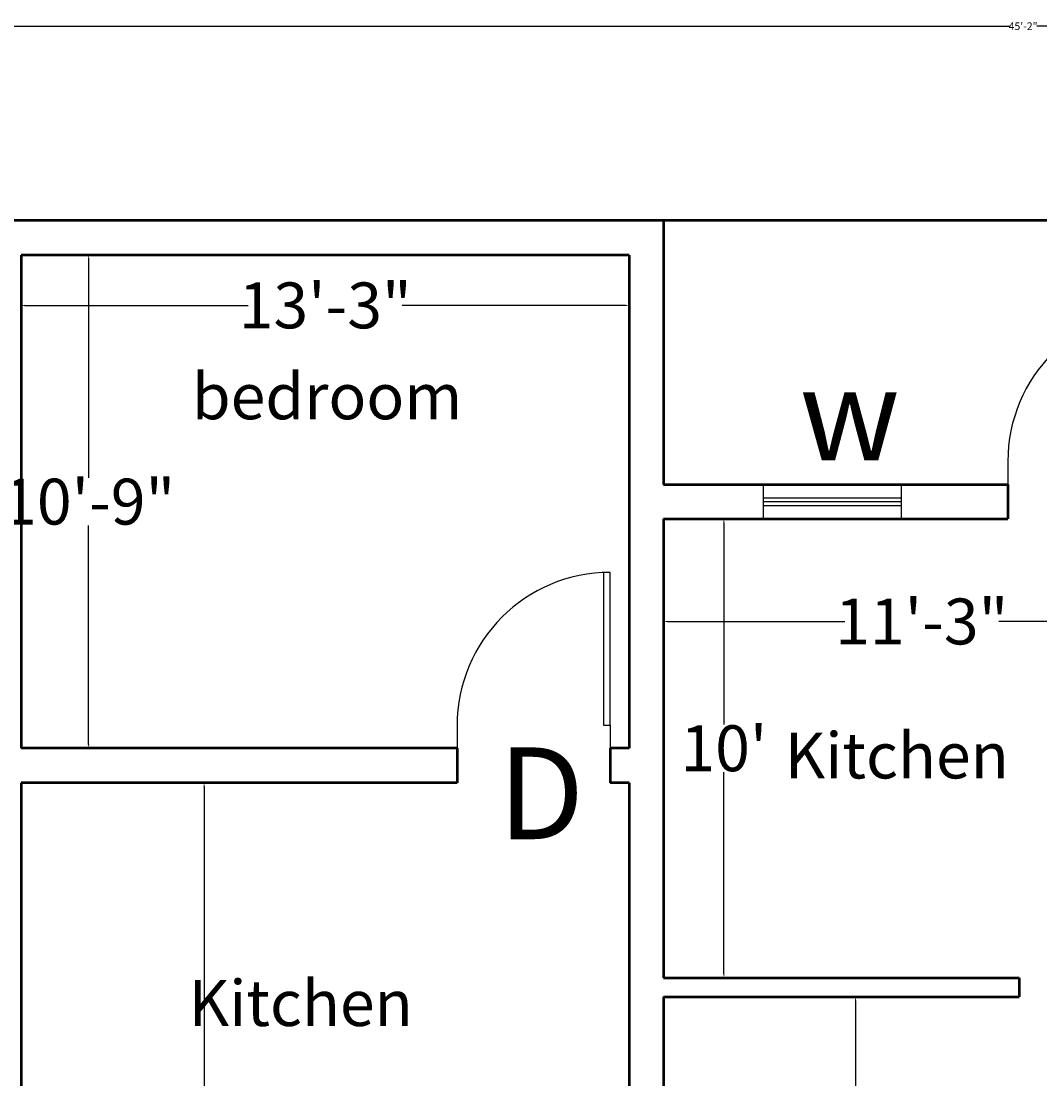
# Model space of a CAD drawing. Units: inches. Extents: x 409 to 7572, y 7 to 725.
# Tile 17 of 38: x 2984 to 3250, y 448 to 725. Entities that reach past the tile are written whole.
import ezdxf

# ---------------------------------------------------------------- set-up
doc = ezdxf.new("R2010")
doc.units = ezdxf.units.IN
doc.header["$MEASUREMENT"] = 0
for name, color, linetype, lineweight in [('A-ANNO-DIMS', 2, 'Continuous', 18), ('A-ANNO-SYMB', 3, 'Continuous', 25), ('A-AREA-IDEN', 7, 'Continuous', 25), ('A-DOOR', 3, 'Continuous', 25), ('A-GLAZ', 4, 'Continuous', 25), ('A-WALL', 7, 'Continuous', 50)]:
    doc.layers.add(name, color=color, linetype=linetype, lineweight=lineweight)
doc.styles.get("Standard").update_dxf_attribs({"font": 'arial.ttf'})
doc.dimstyles.get("Standard").update_dxf_attribs({"dimtxt": 2, "dimasz": 1, "dimexe": 0.18, "dimexo": 0.0625, "dimgap": 0.09, "dimtad": 0, "dimtih": 1, "dimtoh": 1, "dimdec": 0, "dimzin": 0, "dimdsep": 46, "dimlunit": 3, "dimtxsty": 'Standard', "dimcen": 0.09, "dimadec": 0, "dimazin": 0, "dimtfac": 1, "dimtdec": 0, "dimtofl": 0, "dimtmove": 0, "dimatfit": 3, "dimfxl": 1, "dimtolj": 1, "dimtzin": 0, "dimarcsym": 0})

# ---------------------------------------------------------------- blocks, each defined once
blk = doc.blocks.new('*U2')
for p, q in [((0, 0), (0, -6)), ((-40, 0), (-40, -6))]:
    blk.add_line(p, q)
blk.add_lwpolyline([(0, 0), (0, 40), (-1.75, 40), (-1.75, 0)], close=True)
blk.add_arc((0, 0), 40, 90, 180)
blk = doc.blocks.new('*D71')
at = {"layer": 'A-ANNO-DIMS', "color": 0, "lineweight": -2, "transparency": 16777216}
for p, q in [((2984.16, 663.53), (3001.93, 663.53)), ((3001.75, 662.53), (3001.75, 605.25)), ((3001.75, 535.53), (3001.75, 592.81)), ((2984.16, 534.53), (3001.93, 534.53))]:
    blk.add_line(p, q, dxfattribs=at)
at = {"layer": 'A-ANNO-DIMS', "color": 0, "transparency": 16777216}
for points in [[(3001.58, 662.53), (3001.92, 662.53), (3001.75, 663.53)], [(3001.58, 535.53), (3001.92, 535.53), (3001.75, 534.53)]]:
    blk.add_solid(points, dxfattribs=at)
at = {"layer": 'DEFPOINTS', "color": 0, "transparency": 16777216}
for p in [(2984.1, 663.53), (2984.1, 534.53), (3001.75, 534.53)]:
    blk.add_point(p, dxfattribs=at)
at = {"layer": 'A-ANNO-DIMS', "color": 0, "transparency": 16777216, "insert": (3001.75, 599.03), "char_height": 2, "attachment_point": 5}
blk.add_mtext('\\A1;{\\H6x;10\'-9"}', dxfattribs=at)
blk = doc.blocks.new('*D72')
at = {"layer": 'A-ANNO-DIMS', "color": 0, "lineweight": -2, "transparency": 16777216}
for p, q in [((2984.1, 663.47), (2984.1, 650.17)), ((3143.1, 663.47), (3143.1, 650.17)), ((2985.1, 650.35), (3043.46, 650.35)), ((3142.1, 650.35), (3083.73, 650.35))]:
    blk.add_line(p, q, dxfattribs=at)
at = {"layer": 'A-ANNO-DIMS', "color": 0, "transparency": 16777216}
for points in [[(2985.1, 650.52), (2985.1, 650.19), (2984.1, 650.35)], [(3142.1, 650.52), (3142.1, 650.19), (3143.1, 650.35)]]:
    blk.add_solid(points, dxfattribs=at)
at = {"layer": 'DEFPOINTS', "color": 0, "transparency": 16777216}
for p in [(2984.1, 663.53), (3143.1, 663.53), (3143.1, 650.35)]:
    blk.add_point(p, dxfattribs=at)
at = {"layer": 'A-ANNO-DIMS', "color": 0, "transparency": 16777216, "insert": (3063.6, 650.35), "char_height": 2, "attachment_point": 5}
blk.add_mtext('\\A1;{\\H6x;13\'-3"}', dxfattribs=at)
blk = doc.blocks.new('*D81')
at = {"layer": 'A-ANNO-DIMS', "color": 0, "lineweight": -2, "transparency": 16777216}
for p, q in [((3152.16, 594.53), (3168.03, 594.53)), ((3167.85, 593.53), (3167.85, 540.75)), ((3167.85, 475.53), (3167.85, 528.31)), ((3152.16, 474.53), (3168.03, 474.53))]:
    blk.add_line(p, q, dxfattribs=at)
at = {"layer": 'A-ANNO-DIMS', "color": 0, "transparency": 16777216}
for points in [[(3167.69, 593.53), (3168.02, 593.53), (3167.85, 594.53)], [(3167.69, 475.53), (3168.02, 475.53), (3167.85, 474.53)]]:
    blk.add_solid(points, dxfattribs=at)
at = {"layer": 'DEFPOINTS', "color": 0, "transparency": 16777216}
for p in [(3152.1, 594.53), (3152.1, 474.53), (3167.85, 474.53)]:
    blk.add_point(p, dxfattribs=at)
at = {"layer": 'A-ANNO-DIMS', "color": 0, "transparency": 16777216, "insert": (3167.85, 534.53), "char_height": 2, "attachment_point": 5}
blk.add_mtext("\\A1;{\\H6x;10'}", dxfattribs=at)
blk = doc.blocks.new('*D83')
at = {"layer": 'A-ANNO-DIMS', "color": 0, "lineweight": -2, "transparency": 16777216}
for p, q in [((3041.04, 525.53), (3031.75, 525.53)), ((3031.93, 524.53), (3031.93, 428.65)), ((3031.93, 320.53), (3031.93, 416.42)), ((3049.04, 319.53), (3031.75, 319.53))]:
    blk.add_line(p, q, dxfattribs=at)
at = {"layer": 'A-ANNO-DIMS', "color": 0, "transparency": 16777216}
for points in [[(3031.77, 524.53), (3032.1, 524.53), (3031.93, 525.53)], [(3031.77, 320.53), (3032.1, 320.53), (3031.93, 319.53)]]:
    blk.add_solid(points, dxfattribs=at)
at = {"layer": 'DEFPOINTS', "color": 0, "transparency": 16777216}
for p in [(3041.1, 525.53), (3031.93, 319.53), (3049.1, 319.53)]:
    blk.add_point(p, dxfattribs=at)
at = {"layer": 'A-ANNO-DIMS', "color": 0, "transparency": 16777216, "insert": (3031.93, 422.53), "char_height": 2, "attachment_point": 5}
blk.add_mtext('\\A1;{\\H6x;17\'-2"}', dxfattribs=at)
blk = doc.blocks.new('*D79')
at = {"layer": 'A-ANNO-DIMS', "color": 0, "lineweight": -2, "transparency": 16777216}
for p, q in [((3152.1, 563.4), (3152.1, 567.87)), ((3153.1, 567.69), (3199.46, 567.69)), ((3286.1, 567.69), (3239.73, 567.69)), ((3287.1, 563.4), (3287.1, 567.87))]:
    blk.add_line(p, q, dxfattribs=at)
at = {"layer": 'A-ANNO-DIMS', "color": 0, "transparency": 16777216}
for points in [[(3153.1, 567.86), (3153.1, 567.52), (3152.1, 567.69)], [(3286.1, 567.86), (3286.1, 567.52), (3287.1, 567.69)]]:
    blk.add_solid(points, dxfattribs=at)
at = {"layer": 'DEFPOINTS', "color": 0, "transparency": 16777216}
for p in [(3287.1, 567.69), (3152.1, 563.33), (3287.1, 563.33)]:
    blk.add_point(p, dxfattribs=at)
at = {"layer": 'A-ANNO-DIMS', "color": 0, "transparency": 16777216, "insert": (3219.6, 567.69), "char_height": 2, "attachment_point": 5}
blk.add_mtext('\\A1;{\\H6x;11\'-3"}', dxfattribs=at)
blk = doc.blocks.new('*D84')
at = {"layer": 'A-ANNO-DIMS', "color": 0, "lineweight": -2, "transparency": 16777216}
for p, q in [((3206.36, 469.53), (3202.12, 469.53)), ((3202.3, 468.53), (3202.3, 409.65)), ((3202.3, 338.53), (3202.3, 397.42)), ((3207.54, 337.53), (3202.12, 337.53))]:
    blk.add_line(p, q, dxfattribs=at)
at = {"layer": 'A-ANNO-DIMS', "color": 0, "transparency": 16777216}
for points in [[(3202.13, 468.53), (3202.46, 468.53), (3202.3, 469.53)], [(3202.13, 338.53), (3202.46, 338.53), (3202.3, 337.53)]]:
    blk.add_solid(points, dxfattribs=at)
at = {"layer": 'DEFPOINTS', "color": 0, "transparency": 16777216}
for p in [(3206.42, 469.53), (3202.3, 337.53), (3207.6, 337.53)]:
    blk.add_point(p, dxfattribs=at)
at = {"layer": 'A-ANNO-DIMS', "color": 0, "transparency": 16777216, "insert": (3202.3, 403.53), "char_height": 2, "attachment_point": 5}
blk.add_mtext("\\A1;{\\H6x;11'}", dxfattribs=at)
blk = doc.blocks.new('*D90')
at = {"layer": 'A-ANNO-DIMS', "color": 0, "lineweight": -2, "transparency": 16777216}
for p, q in [((2975.1, 672.59), (2975.1, 723.56)), ((2976.1, 723.38), (3242.53, 723.38)), ((3516.1, 723.38), (3249.66, 723.38)), ((3517.1, 672.59), (3517.1, 723.56))]:
    blk.add_line(p, q, dxfattribs=at)
at = {"layer": 'A-ANNO-DIMS', "color": 0, "transparency": 16777216}
for points in [[(2976.1, 723.55), (2976.1, 723.22), (2975.1, 723.38)], [(3516.1, 723.55), (3516.1, 723.22), (3517.1, 723.38)]]:
    blk.add_solid(points, dxfattribs=at)
at = {"layer": 'DEFPOINTS', "color": 0, "transparency": 16777216}
for p in [(2975.1, 723.38), (2975.1, 672.53), (3517.1, 672.53)]:
    blk.add_point(p, dxfattribs=at)
at = {"layer": 'A-ANNO-DIMS', "color": 0, "transparency": 16777216, "insert": (3246.1, 723.38), "char_height": 2, "attachment_point": 5}
blk.add_mtext('\\A1;45\'-2"', dxfattribs=at)
blk = doc.blocks.new('WIN-36')
for p, q in [((1699.82, 514.65), (1699.82, 478.65)), ((1700.82, 514.65), (1700.82, 478.65)), ((1701.82, 514.65), (1701.82, 478.65))]:
    blk.add_line(p, q)
blk.add_lwpolyline([(1705.32, 514.65), (1705.32, 478.65), (1696.32, 478.65), (1696.32, 514.65)], close=True)

msp = doc.modelspace()

# ---------------------------------------------------------------- linework, layer by layer
at = {"layer": 'A-WALL'}
for p, q in [((3517.1, 672.53), (2975.1, 672.53)), ((3152.1, 672.53), (3152.1, 603.53)), ((3143.1, 663.53), (2984.1, 663.53)), ((2984.1, 663.53), (2984.1, 534.53)), ((3143.1, 663.53), (3143.1, 534.53)), ((3143.1, 663.53), (3143.1, 534.53)), ((3152.1, 603.53), (3242.1, 603.53)), ((3242.1, 603.53), (3242.1, 594.53)), ((3152.1, 594.53), (3242.1, 594.53)), ((3152.1, 594.53), (3152.1, 474.53)), ((3098.1, 534.53), (2984.1, 534.53)), ((3098.1, 534.53), (3098.1, 525.53)), ((3143.1, 534.53), (3138.1, 534.53)), ((3138.1, 534.53), (3138.1, 525.53)), ((3098.1, 525.53), (2984.1, 525.53)), ((2984.1, 525.53), (2984.1, 404.53)), ((3143.1, 525.53), (3138.1, 525.53)), ((3143.1, 525.53), (3143.1, 319.53)), ((3152.1, 474.53), (3245.1, 474.53)), ((3245.1, 474.53), (3245.1, 469.53)), ((3152.1, 469.53), (3245.1, 469.53)), ((3152.1, 469.53), (3152.1, 337.53))]:
    msp.add_line(p, q, dxfattribs=at)

# ---------------------------------------------------------------- block references
at = {"layer": 'A-DOOR'}
for p in [(3282.1, 609.53), (3138.1, 540.53)]:
    msp.add_blockref('*U2', p, dxfattribs=at)
at = {"layer": 'A-GLAZ', "rotation": 89.99999999999905}
msp.add_blockref('WIN-36', (3692.84, -1101.79), dxfattribs=at)

# ---------------------------------------------------------------- texts
at = {"layer": 'A-ANNO-SYMB', "char_height": 24, "attachment_point": 1}
for s, width, insert in [('w', 18.2582, (3187.63, 633.82)), ('D', 19.1972, (3108.82, 534.75))]:
    msp.add_mtext_dynamic_manual_height_columns(s, width=width, gutter_width=1, heights=[0], dxfattribs=dict(at, insert=insert))
at = {"layer": 'A-AREA-IDEN', "char_height": 12, "attachment_point": 1}
for s, width, insert in [('bedroom', 40.9017, (3028.76, 632.57)), ('Kitchen ', 61.5504, (3183.78, 538.64)), ('Kitchen ', 61.5504, (3027.92, 473.89))]:
    msp.add_mtext_dynamic_manual_height_columns(s, width=width, gutter_width=1, heights=[0], dxfattribs=dict(at, insert=insert))

# ---------------------------------------------------------------- dimensions: what is measured, and where the dimension line sits
at = {"layer": 'A-ANNO-DIMS'}
dim = msp.add_linear_dim(base=(2975.1, 723.38), p1=(3517.1, 672.53), p2=(2975.1, 672.53), dimstyle='Standard', override={"dimclrd": 0, "dimclre": 0, "dimclrt": 0}, dxfattribs=at)
dim.commit()
dim.dimension.update_dxf_attribs({"geometry": '*D90', "text_midpoint": (3246.1, 723.38)})
for base, p1, p2, picture, middle in [((3001.75, 534.53), (2984.1, 663.53), (2984.1, 534.53), '*D71', (3001.75, 599.03)), ((3167.85, 474.53), (3152.1, 594.53), (3152.1, 474.53), '*D81', (3167.85, 534.53)), ((3202.3, 337.53), (3206.42, 469.53), (3207.6, 337.53), '*D84', (3202.3, 403.53))]:
    dim = msp.add_linear_dim(base=base, p1=p1, p2=p2, angle=90, text='{\\H6x;<>}', dimstyle='Standard', override={"dimclrd": 0, "dimclre": 0, "dimclrt": 0}, dxfattribs=at)
    dim.commit()
    dim.dimension.update_dxf_attribs({"geometry": picture, "text_midpoint": middle})
for base, p1, p2, picture, middle in [((3143.1, 650.35), (2984.1, 663.53), (3143.1, 663.53), '*D72', (3063.6, 650.35)), ((3287.1, 567.69), (3152.1, 563.33), (3287.1, 563.33), '*D79', (3219.6, 567.69))]:
    dim = msp.add_linear_dim(base=base, p1=p1, p2=p2, text='{\\H6x;<>}', dimstyle='Standard', override={"dimclrd": 0, "dimclre": 0, "dimclrt": 0}, dxfattribs=at)
    dim.commit()
    dim.dimension.update_dxf_attribs({"geometry": picture, "text_midpoint": middle})
dim = msp.add_linear_dim(base=(3031.93, 319.53), p1=(3041.1, 525.53), p2=(3049.1, 319.53), angle=90, text='{\\H6x;<>}', dimstyle='Standard', override={"dimclrd": 0, "dimclre": 0, "dimclrt": 0}, dxfattribs=at)
dim.commit()
dim.dimension.update_dxf_attribs({"geometry": '*D83', "text_midpoint": (3031.93, 422.53), "dimtype": 160})

doc.saveas('drawing.dxf')
